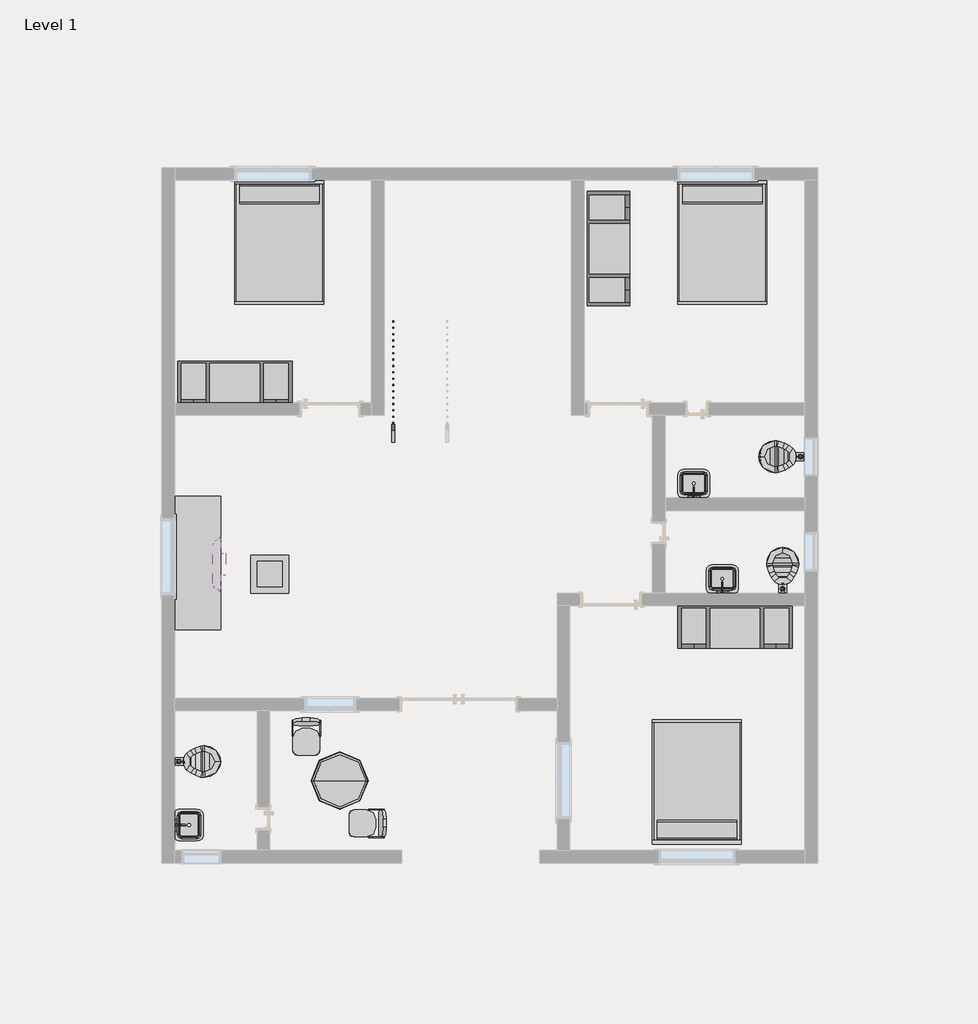
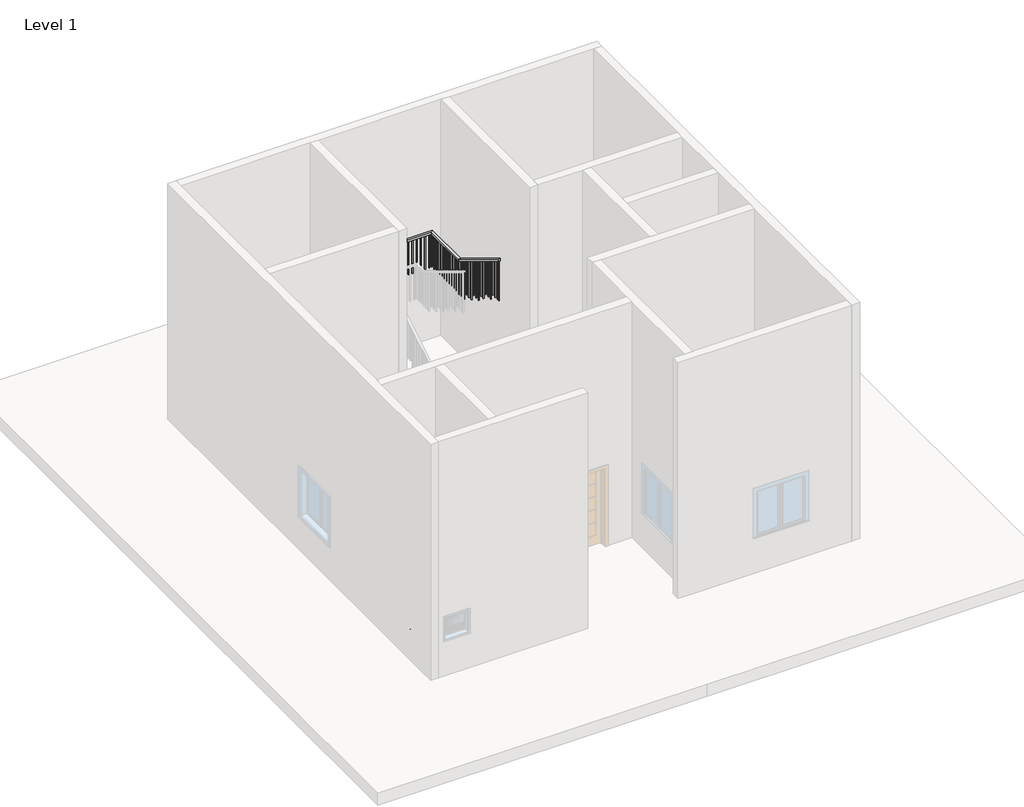
# One storey, part 3 of 3: 12 furniture elements, 6 flow terminals, 1 railing.
"""IFC4 building model written with IfcOpenShell, lengths in millimetres."""

from ifc_helpers import new_model, si_unit, frame, origin, place, context, project, spatial, polyline, outline, extrude, faceted_brep, transform, mapped, element, save
from components import flow_terminal_62a433f7, flow_terminal_bd37145e, furniture_096e7f55, furniture_cf0b6580, furniture_3d1d9cbc, furniture_56245f3a, furniture_b5c51a22, furniture_92191dda, furniture_c80d6d9c

model = new_model("IFC4")

# Units and contexts
model_context = context("Model", 3, world=origin())
ifc_project = project(units=[si_unit("LENGTHUNIT", "METRE", prefix="MILLI")], contexts=[model_context])

# Site, building, storey
site = spatial("IfcSite", under=ifc_project)
building = spatial("IfcBuilding", under=site)
storey = spatial("IfcBuildingStorey", under=building, Name="Level 1", Elevation=0.0)

# Flow terminals
placement = place(None, origin())
flow_terminal_shape = flow_terminal_62a433f7(model_context)
element("IfcFlowTerminal", 1, ObjectType="Sink Vanity-Square : 20\" x 18\"", at=placement, inside=storey, context=model_context, shape_type="MappedRepresentation", body=[
    mapped(flow_terminal_shape, transform((-11513.3414158, 2337.5597862, 0.0), x_axis=(0.0, 1.0000000000000002, 0.0), y_axis=(-1.0000000000000002, 0.0, 0.0), z_axis=(0.0, 0.0, 1.0))),
])
element("IfcFlowTerminal", 2, ObjectType="Sink Vanity-Square : 20\" x 18\"", at=placement, inside=storey, context=model_context, shape_type="MappedRepresentation", body=[
    mapped(flow_terminal_shape, transform((-3371.9975763, 7765.7944279, 0.0), x_axis=(-1.0000000000000004, 0.0, 0.0), y_axis=(0.0, -1.0000000000000004, 0.0), z_axis=(0.0, 0.0, 1.0))),
])
element("IfcFlowTerminal", 3, ObjectType="Sink Vanity-Square : 20\" x 18\"", at=placement, inside=storey, context=model_context, shape_type="MappedRepresentation", body=[
    mapped(flow_terminal_shape, transform((-2914.7975763, 6241.7944279, 0.0), x_axis=(-1.0, 0.0, 0.0), y_axis=(0.0, -1.0, 0.0), z_axis=(0.0, 0.0, 1.0))),
])
flow_terminal_2_shape = flow_terminal_bd37145e(model_context)
element("IfcFlowTerminal", 4, ObjectType="Toilet-Commercial-Wall-3D : 15\" Seat Height", at=placement, inside=storey, context=model_context, shape_type="MappedRepresentation", body=[
    mapped(flow_terminal_2_shape, transform((-1508.0868169, 7841.1458729, 0.0), x_axis=(0.0, 1.0, 0.0), y_axis=(-1.0, 0.0, 0.0), z_axis=(0.0, 0.0, 1.0))),
])
element("IfcFlowTerminal", 5, ObjectType="Toilet-Commercial-Wall-3D : 15\" Seat Height", at=placement, inside=storey, context=model_context, shape_type="MappedRepresentation", body=[
    mapped(flow_terminal_2_shape, transform((-2370.1899707, 5960.0490268, 0.0), x_axis=(1.0, 0.0, 0.0), y_axis=(0.0, 1.0, 0.0), z_axis=(0.0, 0.0, 1.0))),
])
element("IfcFlowTerminal", 6, ObjectType="Toilet-Commercial-Wall-3D : 15\" Seat Height", at=placement, inside=storey, context=model_context, shape_type="MappedRepresentation", body=[
    mapped(flow_terminal_2_shape, transform((-11795.0868169, 3774.1521806, 0.0), x_axis=(0.0, -1.0, 0.0), y_axis=(1.0, 0.0, 0.0), z_axis=(0.0, 0.0, 1.0))),
])

# Furniture
furniture_shape = furniture_096e7f55(model_context)
element("IfcFurniture", 7, ObjectType="Bed-Shaker : Double 56\" x 78\"", at=placement, inside=storey, context=model_context, shape_type="MappedRepresentation", body=[
    mapped(furniture_shape, transform((-9998.0368169, 12665.6490268, 0.0), x_axis=(1.0, 0.0, 0.0), y_axis=(0.0, 1.0, 0.0), z_axis=(0.0, 0.0, 1.0))),
])
element("IfcFurniture", 8, ObjectType="Bed-Shaker : Double 56\" x 78\"", at=placement, inside=storey, context=model_context, shape_type="MappedRepresentation", body=[
    mapped(furniture_shape, transform((-2911.4368169, 12665.6490268, 0.0), x_axis=(1.0, 0.0, 0.0), y_axis=(0.0, 1.0, 0.0), z_axis=(0.0, 0.0, 1.0))),
])
element("IfcFurniture", 9, ObjectType="Bed-Shaker : Double 56\" x 78\"", at=placement, inside=storey, context=model_context, shape_type="MappedRepresentation", body=[
    mapped(furniture_shape, transform((-3355.9368169, 2056.4587448, 0.0), x_axis=(-1.0, 0.0, 0.0), y_axis=(0.0, -1.0, 0.0), z_axis=(0.0, 0.0, 1.0))),
])
furniture_2_shape = furniture_cf0b6580(model_context)
element("IfcFurniture", 10, ObjectType="Entertainment Center : 72\" x 72\" x 24\"", at=placement, inside=storey, context=model_context, shape_type="MappedRepresentation", body=[
    mapped(furniture_2_shape, transform((-10728.2868169, 9871.6490268, 0.0), x_axis=(1.0, 0.0, 0.0), y_axis=(0.0, 1.0, 0.0), z_axis=(0.0, 0.0, 1.0))),
])
element("IfcFurniture", 11, ObjectType="Entertainment Center : 72\" x 72\" x 24\"", at=placement, inside=storey, context=model_context, shape_type="MappedRepresentation", body=[
    mapped(furniture_2_shape, transform((-5191.0868169, 11573.4490268, 0.0), x_axis=(0.0, 1.0, 0.0), y_axis=(-1.0, 0.0, 0.0), z_axis=(0.0, 0.0, 1.0))),
])
element("IfcFurniture", 12, ObjectType="Entertainment Center : 72\" x 72\" x 24\"", at=placement, inside=storey, context=model_context, shape_type="MappedRepresentation", body=[
    mapped(furniture_2_shape, transform((-2727.2868169, 5960.0490268, 0.0), x_axis=(1.0, 0.0, 0.0), y_axis=(0.0, 1.0, 0.0), z_axis=(0.0, 0.0, 1.0))),
])
furniture_3_shape = furniture_3d1d9cbc(model_context)
element("IfcFurniture", 13, ObjectType="Seating-Auditorium : 18\" x 24\" x 30\"", at=placement, inside=storey, context=model_context, shape_type="MappedRepresentation", body=[
    mapped(furniture_3_shape, transform((-9424.558948, 3965.5244366, 0.0), x_axis=(-1.0000000000000009, 0.0, 0.0), y_axis=(0.0, -1.0000000000000009, 0.0), z_axis=(0.0, 0.0, 1.0))),
])
element("IfcFurniture", 14, ObjectType="Seating-Auditorium : 18\" x 24\" x 30\"", at=placement, inside=storey, context=model_context, shape_type="MappedRepresentation", body=[
    mapped(furniture_3_shape, transform((-8404.811407, 2217.9211579, 0.0), x_axis=(0.0, 1.0000000000000004, 0.0), y_axis=(-1.0000000000000004, 0.0, 0.0), z_axis=(0.0, 0.0, 1.0))),
])
furniture_4_shape = furniture_56245f3a(model_context)
element("IfcFurniture", 15, ObjectType="TV - Flat Screen : 32\"", at=placement, inside=storey, context=model_context, shape_type="MappedRepresentation", body=[
    mapped(furniture_4_shape, transform((-11026.3147399, 6526.0559822, 1219.2), x_axis=(0.0, 1.0000000000000009, 0.0), y_axis=(-1.0000000000000009, 0.0, 0.0), z_axis=(0.0, 0.0, 1.0))),
])
furniture_5_shape = furniture_b5c51a22(model_context)
element("IfcFurniture", 16, ObjectType="Table-Coffee : 24\" x 24\" x 24\"", at=placement, inside=storey, context=model_context, shape_type="MappedRepresentation", body=[
    mapped(furniture_5_shape, transform((-10074.2757391, 6348.1832601, 0.0), x_axis=(0.0, 1.0000000000000002, 0.0), y_axis=(-1.0000000000000002, 0.0, 0.0), z_axis=(0.0, 0.0, 1.0))),
])
furniture_6_shape = furniture_92191dda(model_context)
element("IfcFurniture", 17, ObjectType="Table-Dining : 30\" x 84\" x 22\"", at=placement, inside=storey, context=model_context, shape_type="MappedRepresentation", body=[
    mapped(furniture_6_shape, transform((-11242.6757391, 6525.9832601, 0.0), x_axis=(0.0, 1.0, 0.0), y_axis=(-1.0, 0.0, 0.0), z_axis=(0.0, 0.0, 1.0))),
])
furniture_7_shape = furniture_c80d6d9c(model_context)
element("IfcFurniture", 18, ObjectType="Table-Round : 36\" Diameter", at=placement, inside=storey, context=model_context, shape_type="MappedRepresentation", body=[
    mapped(furniture_7_shape, transform((-9051.8868169, 3064.4490268, 0.0), x_axis=(1.0, 0.0, 0.0), y_axis=(0.0, 1.0, 0.0), z_axis=(0.0, 0.0, 1.0))),
])

# Railing
element("IfcRailing", 19, ObjectType="Handrail - Rectangular", at=placement, inside=storey, context=model_context, shape_type="SolidModel", body=[
    faceted_brep([(-8219.6582637, 8478.2414332, 1083.7333333), (-8219.6582637, 8478.2414332, 1024.3318731), (-8168.8582637, 8478.2414332, 1024.3318731), (-8168.8582637, 8478.2414332, 1083.7333333), (-8219.6582637, 11551.6414332, 2946.4), (-8219.6582637, 11565.8338426, 2895.6), (-8168.8582637, 11565.8338426, 2895.6), (-8168.8582637, 11551.6414332, 2946.4), (-8219.6582637, 12466.0414332, 2946.4), (-8219.6582637, 12466.0414332, 2895.6), (-8168.8582637, 12415.2414332, 2895.6), (-8168.8582637, 12415.2414332, 2946.4), (-5664.5029886, 12466.0414332, 2946.4), (-5664.5029886, 12466.0414332, 2895.6), (-5715.3029886, 12415.2414332, 2895.6), (-5715.3029886, 12415.2414332, 2946.4), (-5664.5029886, 11272.2414332, 2946.4), (-5664.5029886, 11258.0490238, 2895.6), (-5715.3029886, 11258.0490238, 2895.6), (-5715.3029886, 11272.2414332, 2946.4), (-5664.5029886, 9595.8414332, 3962.4), (-5715.3029886, 9595.8414332, 3962.4), (-5715.3029886, 9595.8414332, 3902.9985397), (-5664.5029886, 9595.8414332, 3902.9985397)], [[[0, 1, 2, 3]], [[1, 0, 4, 5]], [[2, 1, 5, 6]], [[3, 2, 6, 7]], [[0, 3, 7, 4]], [[5, 4, 8, 9]], [[6, 5, 9, 10]], [[7, 6, 10, 11]], [[4, 7, 11, 8]], [[9, 8, 12, 13]], [[10, 9, 13, 14]], [[11, 10, 14, 15]], [[8, 11, 15, 12]], [[13, 12, 16, 17]], [[14, 13, 17, 18]], [[15, 14, 18, 19]], [[12, 15, 19, 16]], [[20, 21, 22, 23]], [[17, 16, 20, 23]], [[18, 17, 23, 22]], [[19, 18, 22, 21]], [[16, 19, 21, 20]]]),
    extrude(outline(polyline([(9656.1664332, 3866.4379337), (9656.1664332, 2878.6666667), (9637.1164332, 2878.6666667), (9637.1164332, 3877.9833882), (9656.1664332, 3866.4379337)])), frame((-5699.4279886, 0.0, 0.0), z_axis=(1.0, 0.0, 0.0), x_axis=(0.0, 1.0, 0.0)), (0.0, 0.0, 1.0), 19.05),
    extrude(outline(polyline([(9757.7664332, 3804.8621761), (9757.7664332, 2878.6666667), (9738.7164332, 2878.6666667), (9738.7164332, 3816.4076307), (9757.7664332, 3804.8621761)])), frame((-5699.4279886, 0.0, 0.0), z_axis=(1.0, 0.0, 0.0), x_axis=(0.0, 1.0, 0.0)), (0.0, 0.0, 1.0), 19.05),
    extrude(outline(polyline([(9859.3664332, 3743.2864185), (9859.3664332, 2878.6666667), (9840.3164332, 2878.6666667), (9840.3164332, 3754.8318731), (9859.3664332, 3743.2864185)])), frame((-5699.4279886, 0.0, 0.0), z_axis=(1.0, 0.0, 0.0), x_axis=(0.0, 1.0, 0.0)), (0.0, 0.0, 1.0), 19.05),
    extrude(outline(polyline([(9960.9664332, 3681.710661), (9960.9664332, 2709.3333333), (9941.9164332, 2709.3333333), (9941.9164332, 3693.2561155), (9960.9664332, 3681.710661)])), frame((-5699.4279886, 0.0, 0.0), z_axis=(1.0, 0.0, 0.0), x_axis=(0.0, 1.0, 0.0)), (0.0, 0.0, 1.0), 19.05),
    extrude(outline(polyline([(10062.5664332, 3620.1349034), (10062.5664332, 2709.3333333), (10043.5164332, 2709.3333333), (10043.5164332, 3631.6803579), (10062.5664332, 3620.1349034)])), frame((-5699.4279886, 0.0, 0.0), z_axis=(1.0, 0.0, 0.0), x_axis=(0.0, 1.0, 0.0)), (0.0, 0.0, 1.0), 19.05),
    extrude(outline(polyline([(10164.1664332, 3558.5591458), (10164.1664332, 2709.3333333), (10145.1164332, 2709.3333333), (10145.1164332, 3570.1046004), (10164.1664332, 3558.5591458)])), frame((-5699.4279886, 0.0, 0.0), z_axis=(1.0, 0.0, 0.0), x_axis=(0.0, 1.0, 0.0)), (0.0, 0.0, 1.0), 19.05),
    extrude(outline(polyline([(10265.7664332, 3496.9833882), (10265.7664332, 2540.0), (10246.7164332, 2540.0), (10246.7164332, 3508.5288428), (10265.7664332, 3496.9833882)])), frame((-5699.4279886, 0.0, 0.0), z_axis=(1.0, 0.0, 0.0), x_axis=(0.0, 1.0, 0.0)), (0.0, 0.0, 1.0), 19.05),
    extrude(outline(polyline([(10367.3664332, 3435.4076307), (10367.3664332, 2540.0), (10348.3164332, 2540.0), (10348.3164332, 3446.9530852), (10367.3664332, 3435.4076307)])), frame((-5699.4279886, 0.0, 0.0), z_axis=(1.0, 0.0, 0.0), x_axis=(0.0, 1.0, 0.0)), (0.0, 0.0, 1.0), 19.05),
    extrude(outline(polyline([(10468.9664332, 3373.8318731), (10468.9664332, 2370.6666667), (10449.9164332, 2370.6666667), (10449.9164332, 3385.3773276), (10468.9664332, 3373.8318731)])), frame((-5699.4279886, 0.0, 0.0), z_axis=(1.0, 0.0, 0.0), x_axis=(0.0, 1.0, 0.0)), (0.0, 0.0, 1.0), 19.05),
    extrude(outline(polyline([(10570.5664332, 3312.2561155), (10570.5664332, 2370.6666667), (10551.5164332, 2370.6666667), (10551.5164332, 3323.80157), (10570.5664332, 3312.2561155)])), frame((-5699.4279886, 0.0, 0.0), z_axis=(1.0, 0.0, 0.0), x_axis=(0.0, 1.0, 0.0)), (0.0, 0.0, 1.0), 19.05),
    extrude(outline(polyline([(10672.1664332, 3250.6803579), (10672.1664332, 2370.6666667), (10653.1164332, 2370.6666667), (10653.1164332, 3262.2258125), (10672.1664332, 3250.6803579)])), frame((-5699.4279886, 0.0, 0.0), z_axis=(1.0, 0.0, 0.0), x_axis=(0.0, 1.0, 0.0)), (0.0, 0.0, 1.0), 19.05),
    extrude(outline(polyline([(10773.7664332, 3189.1046004), (10773.7664332, 2201.3333333), (10754.7164332, 2201.3333333), (10754.7164332, 3200.6500549), (10773.7664332, 3189.1046004)])), frame((-5699.4279886, 0.0, 0.0), z_axis=(1.0, 0.0, 0.0), x_axis=(0.0, 1.0, 0.0)), (0.0, 0.0, 1.0), 19.05),
    extrude(outline(polyline([(10875.3664332, 3127.5288428), (10875.3664332, 2201.3333333), (10856.3164332, 2201.3333333), (10856.3164332, 3139.0742973), (10875.3664332, 3127.5288428)])), frame((-5699.4279886, 0.0, 0.0), z_axis=(1.0, 0.0, 0.0), x_axis=(0.0, 1.0, 0.0)), (0.0, 0.0, 1.0), 19.05),
    extrude(outline(polyline([(10976.9664332, 3065.9530852), (10976.9664332, 2201.3333333), (10957.9164332, 2201.3333333), (10957.9164332, 3077.4985397), (10976.9664332, 3065.9530852)])), frame((-5699.4279886, 0.0, 0.0), z_axis=(1.0, 0.0, 0.0), x_axis=(0.0, 1.0, 0.0)), (0.0, 0.0, 1.0), 19.05),
    extrude(outline(polyline([(11078.5664332, 3004.3773276), (11078.5664332, 2032.0), (11059.5164332, 2032.0), (11059.5164332, 3015.9227822), (11078.5664332, 3004.3773276)])), frame((-5699.4279886, 0.0, 0.0), z_axis=(1.0, 0.0, 0.0), x_axis=(0.0, 1.0, 0.0)), (0.0, 0.0, 1.0), 19.05),
    extrude(outline(polyline([(11180.1664332, 2942.80157), (11180.1664332, 2032.0), (11161.1164332, 2032.0), (11161.1164332, 2954.3470246), (11180.1664332, 2942.80157)])), frame((-5699.4279886, 0.0, 0.0), z_axis=(1.0, 0.0, 0.0), x_axis=(0.0, 1.0, 0.0)), (0.0, 0.0, 1.0), 19.05),
    extrude(outline(polyline([(-5680.3779886, 11332.5664332), (-5680.3779886, 11313.5164332), (-5699.4279886, 11313.5164332), (-5699.4279886, 11332.5664332), (-5680.3779886, 11332.5664332)])), frame((0.0, 0.0, 2032.0), z_axis=(0.0, 0.0, 1.0), x_axis=(1.0, 0.0, 0.0)), (0.0, 0.0, 1.0), 863.6),
    extrude(outline(polyline([(-5680.3779886, 11434.1664332), (-5680.3779886, 11415.1164332), (-5699.4279886, 11415.1164332), (-5699.4279886, 11434.1664332), (-5680.3779886, 11434.1664332)])), frame((0.0, 0.0, 2032.0), z_axis=(0.0, 0.0, 1.0), x_axis=(1.0, 0.0, 0.0)), (0.0, 0.0, 1.0), 863.6),
    extrude(outline(polyline([(-5680.3779886, 11535.7664332), (-5680.3779886, 11516.7164332), (-5699.4279886, 11516.7164332), (-5699.4279886, 11535.7664332), (-5680.3779886, 11535.7664332)])), frame((0.0, 0.0, 2032.0), z_axis=(0.0, 0.0, 1.0), x_axis=(1.0, 0.0, 0.0)), (0.0, 0.0, 1.0), 863.6),
    extrude(outline(polyline([(-5680.3779886, 11637.3664332), (-5680.3779886, 11618.3164332), (-5699.4279886, 11618.3164332), (-5699.4279886, 11637.3664332), (-5680.3779886, 11637.3664332)])), frame((0.0, 0.0, 2032.0), z_axis=(0.0, 0.0, 1.0), x_axis=(1.0, 0.0, 0.0)), (0.0, 0.0, 1.0), 863.6),
    extrude(outline(polyline([(-5680.3779886, 11738.9664332), (-5680.3779886, 11719.9164332), (-5699.4279886, 11719.9164332), (-5699.4279886, 11738.9664332), (-5680.3779886, 11738.9664332)])), frame((0.0, 0.0, 2032.0), z_axis=(0.0, 0.0, 1.0), x_axis=(1.0, 0.0, 0.0)), (0.0, 0.0, 1.0), 863.6),
    extrude(outline(polyline([(-5680.3779886, 11840.5664332), (-5680.3779886, 11821.5164332), (-5699.4279886, 11821.5164332), (-5699.4279886, 11840.5664332), (-5680.3779886, 11840.5664332)])), frame((0.0, 0.0, 2032.0), z_axis=(0.0, 0.0, 1.0), x_axis=(1.0, 0.0, 0.0)), (0.0, 0.0, 1.0), 863.6),
    extrude(outline(polyline([(-5680.3779886, 11942.1664332), (-5680.3779886, 11923.1164332), (-5699.4279886, 11923.1164332), (-5699.4279886, 11942.1664332), (-5680.3779886, 11942.1664332)])), frame((0.0, 0.0, 2032.0), z_axis=(0.0, 0.0, 1.0), x_axis=(1.0, 0.0, 0.0)), (0.0, 0.0, 1.0), 863.6),
    extrude(outline(polyline([(-5680.3779886, 12043.7664332), (-5680.3779886, 12024.7164332), (-5699.4279886, 12024.7164332), (-5699.4279886, 12043.7664332), (-5680.3779886, 12043.7664332)])), frame((0.0, 0.0, 2032.0), z_axis=(0.0, 0.0, 1.0), x_axis=(1.0, 0.0, 0.0)), (0.0, 0.0, 1.0), 863.6),
    extrude(outline(polyline([(-5680.3779886, 12145.3664332), (-5680.3779886, 12126.3164332), (-5699.4279886, 12126.3164332), (-5699.4279886, 12145.3664332), (-5680.3779886, 12145.3664332)])), frame((0.0, 0.0, 2032.0), z_axis=(0.0, 0.0, 1.0), x_axis=(1.0, 0.0, 0.0)), (0.0, 0.0, 1.0), 863.6),
    extrude(outline(polyline([(-5680.3779886, 12246.9664332), (-5680.3779886, 12227.9164332), (-5699.4279886, 12227.9164332), (-5699.4279886, 12246.9664332), (-5680.3779886, 12246.9664332)])), frame((0.0, 0.0, 2032.0), z_axis=(0.0, 0.0, 1.0), x_axis=(1.0, 0.0, 0.0)), (0.0, 0.0, 1.0), 863.6),
    extrude(outline(polyline([(-5680.3779886, 12348.5664332), (-5680.3779886, 12329.5164332), (-5699.4279886, 12329.5164332), (-5699.4279886, 12348.5664332), (-5680.3779886, 12348.5664332)])), frame((0.0, 0.0, 2032.0), z_axis=(0.0, 0.0, 1.0), x_axis=(1.0, 0.0, 0.0)), (0.0, 0.0, 1.0), 863.6),
    extrude(outline(polyline([(-5765.3832637, 12450.1664332), (-5746.3332637, 12450.1664332), (-5746.3332637, 12431.1164332), (-5765.3832637, 12431.1164332), (-5765.3832637, 12450.1664332)])), frame((0.0, 0.0, 2032.0), z_axis=(0.0, 0.0, 1.0), x_axis=(1.0, 0.0, 0.0)), (0.0, 0.0, 1.0), 863.6),
    extrude(outline(polyline([(-5866.9832637, 12450.1664332), (-5847.9332637, 12450.1664332), (-5847.9332637, 12431.1164332), (-5866.9832637, 12431.1164332), (-5866.9832637, 12450.1664332)])), frame((0.0, 0.0, 2032.0), z_axis=(0.0, 0.0, 1.0), x_axis=(1.0, 0.0, 0.0)), (0.0, 0.0, 1.0), 863.6),
    extrude(outline(polyline([(-5968.5832637, 12450.1664332), (-5949.5332637, 12450.1664332), (-5949.5332637, 12431.1164332), (-5968.5832637, 12431.1164332), (-5968.5832637, 12450.1664332)])), frame((0.0, 0.0, 2032.0), z_axis=(0.0, 0.0, 1.0), x_axis=(1.0, 0.0, 0.0)), (0.0, 0.0, 1.0), 863.6),
    extrude(outline(polyline([(-6070.1832637, 12450.1664332), (-6051.1332637, 12450.1664332), (-6051.1332637, 12431.1164332), (-6070.1832637, 12431.1164332), (-6070.1832637, 12450.1664332)])), frame((0.0, 0.0, 2032.0), z_axis=(0.0, 0.0, 1.0), x_axis=(1.0, 0.0, 0.0)), (0.0, 0.0, 1.0), 863.6),
    extrude(outline(polyline([(-6171.7832637, 12450.1664332), (-6152.7332637, 12450.1664332), (-6152.7332637, 12431.1164332), (-6171.7832637, 12431.1164332), (-6171.7832637, 12450.1664332)])), frame((0.0, 0.0, 2032.0), z_axis=(0.0, 0.0, 1.0), x_axis=(1.0, 0.0, 0.0)), (0.0, 0.0, 1.0), 863.6),
    extrude(outline(polyline([(-6273.3832637, 12450.1664332), (-6254.3332637, 12450.1664332), (-6254.3332637, 12431.1164332), (-6273.3832637, 12431.1164332), (-6273.3832637, 12450.1664332)])), frame((0.0, 0.0, 2032.0), z_axis=(0.0, 0.0, 1.0), x_axis=(1.0, 0.0, 0.0)), (0.0, 0.0, 1.0), 863.6),
    extrude(outline(polyline([(-6374.9832637, 12450.1664332), (-6355.9332637, 12450.1664332), (-6355.9332637, 12431.1164332), (-6374.9832637, 12431.1164332), (-6374.9832637, 12450.1664332)])), frame((0.0, 0.0, 2032.0), z_axis=(0.0, 0.0, 1.0), x_axis=(1.0, 0.0, 0.0)), (0.0, 0.0, 1.0), 863.6),
    extrude(outline(polyline([(-6476.5832637, 12450.1664332), (-6457.5332637, 12450.1664332), (-6457.5332637, 12431.1164332), (-6476.5832637, 12431.1164332), (-6476.5832637, 12450.1664332)])), frame((0.0, 0.0, 2032.0), z_axis=(0.0, 0.0, 1.0), x_axis=(1.0, 0.0, 0.0)), (0.0, 0.0, 1.0), 863.6),
    extrude(outline(polyline([(-6578.1832637, 12450.1664332), (-6559.1332637, 12450.1664332), (-6559.1332637, 12431.1164332), (-6578.1832637, 12431.1164332), (-6578.1832637, 12450.1664332)])), frame((0.0, 0.0, 2032.0), z_axis=(0.0, 0.0, 1.0), x_axis=(1.0, 0.0, 0.0)), (0.0, 0.0, 1.0), 863.6),
    extrude(outline(polyline([(-6679.7832637, 12450.1664332), (-6660.7332637, 12450.1664332), (-6660.7332637, 12431.1164332), (-6679.7832637, 12431.1164332), (-6679.7832637, 12450.1664332)])), frame((0.0, 0.0, 2032.0), z_axis=(0.0, 0.0, 1.0), x_axis=(1.0, 0.0, 0.0)), (0.0, 0.0, 1.0), 863.6),
    extrude(outline(polyline([(-6781.3832637, 12450.1664332), (-6762.3332637, 12450.1664332), (-6762.3332637, 12431.1164332), (-6781.3832637, 12431.1164332), (-6781.3832637, 12450.1664332)])), frame((0.0, 0.0, 2032.0), z_axis=(0.0, 0.0, 1.0), x_axis=(1.0, 0.0, 0.0)), (0.0, 0.0, 1.0), 863.6),
    extrude(outline(polyline([(-6882.9832637, 12450.1664332), (-6863.9332637, 12450.1664332), (-6863.9332637, 12431.1164332), (-6882.9832637, 12431.1164332), (-6882.9832637, 12450.1664332)])), frame((0.0, 0.0, 2032.0), z_axis=(0.0, 0.0, 1.0), x_axis=(1.0, 0.0, 0.0)), (0.0, 0.0, 1.0), 863.6),
    extrude(outline(polyline([(-6984.5832637, 12450.1664332), (-6965.5332637, 12450.1664332), (-6965.5332637, 12431.1164332), (-6984.5832637, 12431.1164332), (-6984.5832637, 12450.1664332)])), frame((0.0, 0.0, 2032.0), z_axis=(0.0, 0.0, 1.0), x_axis=(1.0, 0.0, 0.0)), (0.0, 0.0, 1.0), 863.6),
    extrude(outline(polyline([(-7086.1832637, 12450.1664332), (-7067.1332637, 12450.1664332), (-7067.1332637, 12431.1164332), (-7086.1832637, 12431.1164332), (-7086.1832637, 12450.1664332)])), frame((0.0, 0.0, 2032.0), z_axis=(0.0, 0.0, 1.0), x_axis=(1.0, 0.0, 0.0)), (0.0, 0.0, 1.0), 863.6),
    extrude(outline(polyline([(-7187.7832637, 12450.1664332), (-7168.7332637, 12450.1664332), (-7168.7332637, 12431.1164332), (-7187.7832637, 12431.1164332), (-7187.7832637, 12450.1664332)])), frame((0.0, 0.0, 2032.0), z_axis=(0.0, 0.0, 1.0), x_axis=(1.0, 0.0, 0.0)), (0.0, 0.0, 1.0), 863.6),
    extrude(outline(polyline([(-7289.3832637, 12450.1664332), (-7270.3332637, 12450.1664332), (-7270.3332637, 12431.1164332), (-7289.3832637, 12431.1164332), (-7289.3832637, 12450.1664332)])), frame((0.0, 0.0, 2032.0), z_axis=(0.0, 0.0, 1.0), x_axis=(1.0, 0.0, 0.0)), (0.0, 0.0, 1.0), 863.6),
    extrude(outline(polyline([(-7390.9832637, 12450.1664332), (-7371.9332637, 12450.1664332), (-7371.9332637, 12431.1164332), (-7390.9832637, 12431.1164332), (-7390.9832637, 12450.1664332)])), frame((0.0, 0.0, 2032.0), z_axis=(0.0, 0.0, 1.0), x_axis=(1.0, 0.0, 0.0)), (0.0, 0.0, 1.0), 863.6),
    extrude(outline(polyline([(-7492.5832637, 12450.1664332), (-7473.5332637, 12450.1664332), (-7473.5332637, 12431.1164332), (-7492.5832637, 12431.1164332), (-7492.5832637, 12450.1664332)])), frame((0.0, 0.0, 2032.0), z_axis=(0.0, 0.0, 1.0), x_axis=(1.0, 0.0, 0.0)), (0.0, 0.0, 1.0), 863.6),
    extrude(outline(polyline([(-7594.1832637, 12450.1664332), (-7575.1332637, 12450.1664332), (-7575.1332637, 12431.1164332), (-7594.1832637, 12431.1164332), (-7594.1832637, 12450.1664332)])), frame((0.0, 0.0, 2032.0), z_axis=(0.0, 0.0, 1.0), x_axis=(1.0, 0.0, 0.0)), (0.0, 0.0, 1.0), 863.6),
    extrude(outline(polyline([(-7695.7832637, 12450.1664332), (-7676.7332637, 12450.1664332), (-7676.7332637, 12431.1164332), (-7695.7832637, 12431.1164332), (-7695.7832637, 12450.1664332)])), frame((0.0, 0.0, 2032.0), z_axis=(0.0, 0.0, 1.0), x_axis=(1.0, 0.0, 0.0)), (0.0, 0.0, 1.0), 863.6),
    extrude(outline(polyline([(-7797.3832637, 12450.1664332), (-7778.3332637, 12450.1664332), (-7778.3332637, 12431.1164332), (-7797.3832637, 12431.1164332), (-7797.3832637, 12450.1664332)])), frame((0.0, 0.0, 2032.0), z_axis=(0.0, 0.0, 1.0), x_axis=(1.0, 0.0, 0.0)), (0.0, 0.0, 1.0), 863.6),
    extrude(outline(polyline([(-7898.9832637, 12450.1664332), (-7879.9332637, 12450.1664332), (-7879.9332637, 12431.1164332), (-7898.9832637, 12431.1164332), (-7898.9832637, 12450.1664332)])), frame((0.0, 0.0, 2032.0), z_axis=(0.0, 0.0, 1.0), x_axis=(1.0, 0.0, 0.0)), (0.0, 0.0, 1.0), 863.6),
    extrude(outline(polyline([(-8000.5832637, 12450.1664332), (-7981.5332637, 12450.1664332), (-7981.5332637, 12431.1164332), (-8000.5832637, 12431.1164332), (-8000.5832637, 12450.1664332)])), frame((0.0, 0.0, 2032.0), z_axis=(0.0, 0.0, 1.0), x_axis=(1.0, 0.0, 0.0)), (0.0, 0.0, 1.0), 863.6),
    extrude(outline(polyline([(-8102.1832637, 12450.1664332), (-8083.1332637, 12450.1664332), (-8083.1332637, 12431.1164332), (-8102.1832637, 12431.1164332), (-8102.1832637, 12450.1664332)])), frame((0.0, 0.0, 2032.0), z_axis=(0.0, 0.0, 1.0), x_axis=(1.0, 0.0, 0.0)), (0.0, 0.0, 1.0), 863.6),
    extrude(outline(polyline([(-8203.7832637, 12354.9164332), (-8203.7832637, 12373.9664332), (-8184.7332637, 12373.9664332), (-8184.7332637, 12354.9164332), (-8203.7832637, 12354.9164332)])), frame((0.0, 0.0, 2032.0), z_axis=(0.0, 0.0, 1.0), x_axis=(1.0, 0.0, 0.0)), (0.0, 0.0, 1.0), 863.6),
    extrude(outline(polyline([(-8203.7832637, 12253.3164332), (-8203.7832637, 12272.3664332), (-8184.7332637, 12272.3664332), (-8184.7332637, 12253.3164332), (-8203.7832637, 12253.3164332)])), frame((0.0, 0.0, 2032.0), z_axis=(0.0, 0.0, 1.0), x_axis=(1.0, 0.0, 0.0)), (0.0, 0.0, 1.0), 863.6),
    extrude(outline(polyline([(-8203.7832637, 12151.7164332), (-8203.7832637, 12170.7664332), (-8184.7332637, 12170.7664332), (-8184.7332637, 12151.7164332), (-8203.7832637, 12151.7164332)])), frame((0.0, 0.0, 2032.0), z_axis=(0.0, 0.0, 1.0), x_axis=(1.0, 0.0, 0.0)), (0.0, 0.0, 1.0), 863.6),
    extrude(outline(polyline([(-8203.7832637, 12050.1164332), (-8203.7832637, 12069.1664332), (-8184.7332637, 12069.1664332), (-8184.7332637, 12050.1164332), (-8203.7832637, 12050.1164332)])), frame((0.0, 0.0, 2032.0), z_axis=(0.0, 0.0, 1.0), x_axis=(1.0, 0.0, 0.0)), (0.0, 0.0, 1.0), 863.6),
    extrude(outline(polyline([(-8203.7832637, 11948.5164332), (-8203.7832637, 11967.5664332), (-8184.7332637, 11967.5664332), (-8184.7332637, 11948.5164332), (-8203.7832637, 11948.5164332)])), frame((0.0, 0.0, 2032.0), z_axis=(0.0, 0.0, 1.0), x_axis=(1.0, 0.0, 0.0)), (0.0, 0.0, 1.0), 863.6),
    extrude(outline(polyline([(-8203.7832637, 11846.9164332), (-8203.7832637, 11865.9664332), (-8184.7332637, 11865.9664332), (-8184.7332637, 11846.9164332), (-8203.7832637, 11846.9164332)])), frame((0.0, 0.0, 2032.0), z_axis=(0.0, 0.0, 1.0), x_axis=(1.0, 0.0, 0.0)), (0.0, 0.0, 1.0), 863.6),
    extrude(outline(polyline([(-8203.7832637, 11745.3164332), (-8203.7832637, 11764.3664332), (-8184.7332637, 11764.3664332), (-8184.7332637, 11745.3164332), (-8203.7832637, 11745.3164332)])), frame((0.0, 0.0, 2032.0), z_axis=(0.0, 0.0, 1.0), x_axis=(1.0, 0.0, 0.0)), (0.0, 0.0, 1.0), 863.6),
    extrude(outline(polyline([(-8203.7832637, 11643.7164332), (-8203.7832637, 11662.7664332), (-8184.7332637, 11662.7664332), (-8184.7332637, 11643.7164332), (-8203.7832637, 11643.7164332)])), frame((0.0, 0.0, 2032.0), z_axis=(0.0, 0.0, 1.0), x_axis=(1.0, 0.0, 0.0)), (0.0, 0.0, 1.0), 863.6),
    extrude(outline(polyline([(11535.7664332, 2877.3773276), (11535.7664332, 1862.6666667), (11516.7164332, 1862.6666667), (11516.7164332, 2865.8318731), (11535.7664332, 2877.3773276)])), frame((-8203.7832637, 0.0, 0.0), z_axis=(1.0, 0.0, 0.0), x_axis=(0.0, 1.0, 0.0)), (0.0, 0.0, 1.0), 19.05),
    extrude(outline(polyline([(11434.1664332, 2815.80157), (11434.1664332, 1862.6666667), (11415.1164332, 1862.6666667), (11415.1164332, 2804.2561155), (11434.1664332, 2815.80157)])), frame((-8203.7832637, 0.0, 0.0), z_axis=(1.0, 0.0, 0.0), x_axis=(0.0, 1.0, 0.0)), (0.0, 0.0, 1.0), 19.05),
    extrude(outline(polyline([(11332.5664332, 2754.2258125), (11332.5664332, 1862.6666667), (11313.5164332, 1862.6666667), (11313.5164332, 2742.6803579), (11332.5664332, 2754.2258125)])), frame((-8203.7832637, 0.0, 0.0), z_axis=(1.0, 0.0, 0.0), x_axis=(0.0, 1.0, 0.0)), (0.0, 0.0, 1.0), 19.05),
    extrude(outline(polyline([(11230.9664332, 2692.6500549), (11230.9664332, 1693.3333333), (11211.9164332, 1693.3333333), (11211.9164332, 2681.1046004), (11230.9664332, 2692.6500549)])), frame((-8203.7832637, 0.0, 0.0), z_axis=(1.0, 0.0, 0.0), x_axis=(0.0, 1.0, 0.0)), (0.0, 0.0, 1.0), 19.05),
    extrude(outline(polyline([(11129.3664332, 2631.0742973), (11129.3664332, 1693.3333333), (11110.3164332, 1693.3333333), (11110.3164332, 2619.5288428), (11129.3664332, 2631.0742973)])), frame((-8203.7832637, 0.0, 0.0), z_axis=(1.0, 0.0, 0.0), x_axis=(0.0, 1.0, 0.0)), (0.0, 0.0, 1.0), 19.05),
    extrude(outline(polyline([(11027.7664332, 2569.4985397), (11027.7664332, 1693.3333333), (11008.7164332, 1693.3333333), (11008.7164332, 2557.9530852), (11027.7664332, 2569.4985397)])), frame((-8203.7832637, 0.0, 0.0), z_axis=(1.0, 0.0, 0.0), x_axis=(0.0, 1.0, 0.0)), (0.0, 0.0, 1.0), 19.05),
    extrude(outline(polyline([(10926.1664332, 2507.9227822), (10926.1664332, 1524.0), (10907.1164332, 1524.0), (10907.1164332, 2496.3773276), (10926.1664332, 2507.9227822)])), frame((-8203.7832637, 0.0, 0.0), z_axis=(1.0, 0.0, 0.0), x_axis=(0.0, 1.0, 0.0)), (0.0, 0.0, 1.0), 19.05),
    extrude(outline(polyline([(10824.5664332, 2446.3470246), (10824.5664332, 1524.0), (10805.5164332, 1524.0), (10805.5164332, 2434.80157), (10824.5664332, 2446.3470246)])), frame((-8203.7832637, 0.0, 0.0), z_axis=(1.0, 0.0, 0.0), x_axis=(0.0, 1.0, 0.0)), (0.0, 0.0, 1.0), 19.05),
    extrude(outline(polyline([(10722.9664332, 2384.771267), (10722.9664332, 1524.0), (10703.9164332, 1524.0), (10703.9164332, 2373.2258125), (10722.9664332, 2384.771267)])), frame((-8203.7832637, 0.0, 0.0), z_axis=(1.0, 0.0, 0.0), x_axis=(0.0, 1.0, 0.0)), (0.0, 0.0, 1.0), 19.05),
    extrude(outline(polyline([(10621.3664332, 2323.1955094), (10621.3664332, 1354.6666667), (10602.3164332, 1354.6666667), (10602.3164332, 2311.6500549), (10621.3664332, 2323.1955094)])), frame((-8203.7832637, 0.0, 0.0), z_axis=(1.0, 0.0, 0.0), x_axis=(0.0, 1.0, 0.0)), (0.0, 0.0, 1.0), 19.05),
    extrude(outline(polyline([(10519.7664332, 2261.6197519), (10519.7664332, 1354.6666667), (10500.7164332, 1354.6666667), (10500.7164332, 2250.0742973), (10519.7664332, 2261.6197519)])), frame((-8203.7832637, 0.0, 0.0), z_axis=(1.0, 0.0, 0.0), x_axis=(0.0, 1.0, 0.0)), (0.0, 0.0, 1.0), 19.05),
    extrude(outline(polyline([(10418.1664332, 2200.0439943), (10418.1664332, 1185.3333333), (10399.1164332, 1185.3333333), (10399.1164332, 2188.4985397), (10418.1664332, 2200.0439943)])), frame((-8203.7832637, 0.0, 0.0), z_axis=(1.0, 0.0, 0.0), x_axis=(0.0, 1.0, 0.0)), (0.0, 0.0, 1.0), 19.05),
    extrude(outline(polyline([(10316.5664332, 2138.4682367), (10316.5664332, 1185.3333333), (10297.5164332, 1185.3333333), (10297.5164332, 2126.9227822), (10316.5664332, 2138.4682367)])), frame((-8203.7832637, 0.0, 0.0), z_axis=(1.0, 0.0, 0.0), x_axis=(0.0, 1.0, 0.0)), (0.0, 0.0, 1.0), 19.05),
    extrude(outline(polyline([(10214.9664332, 2076.8924791), (10214.9664332, 1185.3333333), (10195.9164332, 1185.3333333), (10195.9164332, 2065.3470246), (10214.9664332, 2076.8924791)])), frame((-8203.7832637, 0.0, 0.0), z_axis=(1.0, 0.0, 0.0), x_axis=(0.0, 1.0, 0.0)), (0.0, 0.0, 1.0), 19.05),
    extrude(outline(polyline([(10113.3664332, 2015.3167216), (10113.3664332, 1016.0), (10094.3164332, 1016.0), (10094.3164332, 2003.771267), (10113.3664332, 2015.3167216)])), frame((-8203.7832637, 0.0, 0.0), z_axis=(1.0, 0.0, 0.0), x_axis=(0.0, 1.0, 0.0)), (0.0, 0.0, 1.0), 19.05),
    extrude(outline(polyline([(10011.7664332, 1953.740964), (10011.7664332, 1016.0), (9992.7164332, 1016.0), (9992.7164332, 1942.1955094), (10011.7664332, 1953.740964)])), frame((-8203.7832637, 0.0, 0.0), z_axis=(1.0, 0.0, 0.0), x_axis=(0.0, 1.0, 0.0)), (0.0, 0.0, 1.0), 19.05),
    extrude(outline(polyline([(9910.1664332, 1892.1652064), (9910.1664332, 1016.0), (9891.1164332, 1016.0), (9891.1164332, 1880.6197519), (9910.1664332, 1892.1652064)])), frame((-8203.7832637, 0.0, 0.0), z_axis=(1.0, 0.0, 0.0), x_axis=(0.0, 1.0, 0.0)), (0.0, 0.0, 1.0), 19.05),
    extrude(outline(polyline([(9808.5664332, 1830.5894488), (9808.5664332, 846.6666667), (9789.5164332, 846.6666667), (9789.5164332, 1819.0439943), (9808.5664332, 1830.5894488)])), frame((-8203.7832637, 0.0, 0.0), z_axis=(1.0, 0.0, 0.0), x_axis=(0.0, 1.0, 0.0)), (0.0, 0.0, 1.0), 19.05),
    extrude(outline(polyline([(9706.9664332, 1769.0136913), (9706.9664332, 846.6666667), (9687.9164332, 846.6666667), (9687.9164332, 1757.4682367), (9706.9664332, 1769.0136913)])), frame((-8203.7832637, 0.0, 0.0), z_axis=(1.0, 0.0, 0.0), x_axis=(0.0, 1.0, 0.0)), (0.0, 0.0, 1.0), 19.05),
    extrude(outline(polyline([(9605.3664332, 1707.4379337), (9605.3664332, 846.6666667), (9586.3164332, 846.6666667), (9586.3164332, 1695.8924791), (9605.3664332, 1707.4379337)])), frame((-8203.7832637, 0.0, 0.0), z_axis=(1.0, 0.0, 0.0), x_axis=(0.0, 1.0, 0.0)), (0.0, 0.0, 1.0), 19.05),
    extrude(outline(polyline([(9503.7664332, 1645.8621761), (9503.7664332, 677.3333333), (9484.7164332, 677.3333333), (9484.7164332, 1634.3167216), (9503.7664332, 1645.8621761)])), frame((-8203.7832637, 0.0, 0.0), z_axis=(1.0, 0.0, 0.0), x_axis=(0.0, 1.0, 0.0)), (0.0, 0.0, 1.0), 19.05),
    extrude(outline(polyline([(9402.1664332, 1584.2864185), (9402.1664332, 677.3333333), (9383.1164332, 677.3333333), (9383.1164332, 1572.740964), (9402.1664332, 1584.2864185)])), frame((-8203.7832637, 0.0, 0.0), z_axis=(1.0, 0.0, 0.0), x_axis=(0.0, 1.0, 0.0)), (0.0, 0.0, 1.0), 19.05),
    extrude(outline(polyline([(9300.5664332, 1522.710661), (9300.5664332, 508.0), (9281.5164332, 508.0), (9281.5164332, 1511.1652064), (9300.5664332, 1522.710661)])), frame((-8203.7832637, 0.0, 0.0), z_axis=(1.0, 0.0, 0.0), x_axis=(0.0, 1.0, 0.0)), (0.0, 0.0, 1.0), 19.05),
    extrude(outline(polyline([(9198.9664332, 1461.1349034), (9198.9664332, 508.0), (9179.9164332, 508.0), (9179.9164332, 1449.5894488), (9198.9664332, 1461.1349034)])), frame((-8203.7832637, 0.0, 0.0), z_axis=(1.0, 0.0, 0.0), x_axis=(0.0, 1.0, 0.0)), (0.0, 0.0, 1.0), 19.05),
    extrude(outline(polyline([(9097.3664332, 1399.5591458), (9097.3664332, 508.0), (9078.3164332, 508.0), (9078.3164332, 1388.0136913), (9097.3664332, 1399.5591458)])), frame((-8203.7832637, 0.0, 0.0), z_axis=(1.0, 0.0, 0.0), x_axis=(0.0, 1.0, 0.0)), (0.0, 0.0, 1.0), 19.05),
    extrude(outline(polyline([(8995.7664332, 1337.9833882), (8995.7664332, 338.6666667), (8976.7164332, 338.6666667), (8976.7164332, 1326.4379337), (8995.7664332, 1337.9833882)])), frame((-8203.7832637, 0.0, 0.0), z_axis=(1.0, 0.0, 0.0), x_axis=(0.0, 1.0, 0.0)), (0.0, 0.0, 1.0), 19.05),
    extrude(outline(polyline([(8894.1664332, 1276.4076307), (8894.1664332, 338.6666667), (8875.1164332, 338.6666667), (8875.1164332, 1264.8621761), (8894.1664332, 1276.4076307)])), frame((-8203.7832637, 0.0, 0.0), z_axis=(1.0, 0.0, 0.0), x_axis=(0.0, 1.0, 0.0)), (0.0, 0.0, 1.0), 19.05),
    extrude(outline(polyline([(8792.5664332, 1214.8318731), (8792.5664332, 338.6666667), (8773.5164332, 338.6666667), (8773.5164332, 1203.2864185), (8792.5664332, 1214.8318731)])), frame((-8203.7832637, 0.0, 0.0), z_axis=(1.0, 0.0, 0.0), x_axis=(0.0, 1.0, 0.0)), (0.0, 0.0, 1.0), 19.05),
    extrude(outline(polyline([(8690.9664332, 1153.2561155), (8690.9664332, 169.3333333), (8671.9164332, 169.3333333), (8671.9164332, 1141.710661), (8690.9664332, 1153.2561155)])), frame((-8203.7832637, 0.0, 0.0), z_axis=(1.0, 0.0, 0.0), x_axis=(0.0, 1.0, 0.0)), (0.0, 0.0, 1.0), 19.05),
    extrude(outline(polyline([(8589.3664332, 1091.6803579), (8589.3664332, 169.3333333), (8570.3164332, 169.3333333), (8570.3164332, 1080.1349034), (8589.3664332, 1091.6803579)])), frame((-8203.7832637, 0.0, 0.0), z_axis=(1.0, 0.0, 0.0), x_axis=(0.0, 1.0, 0.0)), (0.0, 0.0, 1.0), 19.05),
    extrude(outline(polyline([(-5680.3779886, 11281.7664332), (-5680.3779886, 11262.7164332), (-5699.4279886, 11262.7164332), (-5699.4279886, 11281.7664332), (-5680.3779886, 11281.7664332)])), frame((0.0, 0.0, 2032.0), z_axis=(0.0, 0.0, 1.0), x_axis=(1.0, 0.0, 0.0)), (0.0, 0.0, 1.0), 863.6),
    extrude(outline(polyline([(-5699.4279886, 12450.1664332), (-5680.3779886, 12450.1664332), (-5680.3779886, 12431.1164332), (-5699.4279886, 12431.1164332), (-5699.4279886, 12450.1664332)])), frame((0.0, 0.0, 2032.0), z_axis=(0.0, 0.0, 1.0), x_axis=(1.0, 0.0, 0.0)), (0.0, 0.0, 1.0), 863.6),
    extrude(outline(polyline([(-8203.7832637, 12431.1164332), (-8203.7832637, 12450.1664332), (-8184.7332637, 12450.1664332), (-8184.7332637, 12431.1164332), (-8203.7832637, 12431.1164332)])), frame((0.0, 0.0, 2032.0), z_axis=(0.0, 0.0, 1.0), x_axis=(1.0, 0.0, 0.0)), (0.0, 0.0, 1.0), 863.6),
    extrude(outline(polyline([(11561.1664332, 2892.771267), (11561.1664332, 2032.0), (11542.1164332, 2032.0), (11542.1164332, 2881.2258125), (11561.1664332, 2892.771267)])), frame((-8203.7832637, 0.0, 0.0), z_axis=(1.0, 0.0, 0.0), x_axis=(0.0, 1.0, 0.0)), (0.0, 0.0, 1.0), 19.05),
    extrude(outline(polyline([(9614.8914332, 3891.4530852), (9614.8914332, 2878.6666667), (9595.8414332, 2878.6666667), (9595.8414332, 3902.9985397), (9614.8914332, 3891.4530852)])), frame((-5699.4279886, 0.0, 0.0), z_axis=(1.0, 0.0, 0.0), x_axis=(0.0, 1.0, 0.0)), (0.0, 0.0, 1.0), 19.05),
    extrude(outline(polyline([(8497.2914332, 1035.8773276), (8497.2914332, 169.3333333), (8478.2414332, 169.3333333), (8478.2414332, 1024.3318731), (8497.2914332, 1035.8773276)])), frame((-8203.7832637, 0.0, 0.0), z_axis=(1.0, 0.0, 0.0), x_axis=(0.0, 1.0, 0.0)), (0.0, 0.0, 1.0), 19.05),
])

save(model, "model.ifc")

# Revit data of these elements
# Type "Sink Vanity-Square : 20\" x 18\""
#   Assembly Code = "D2010400"
#   Counter Height = 2' - 7"
#   Depth = 1' - 6"
#   Width = 1' - 8"
#   Basin Material = Porcelain, Linen
#   Faucet Material = Steel, Polished
#   Default Elevation = 0
# Type "Toilet-Commercial-Wall-3D : 15\" Seat Height"
#   Assembly Code = "D2010110"
#   Mounting Height = 1' - 3"
#   Piping Material = Steel, Polished
#   Toilet - Bowl Material = Porcelain, Ivory
#   Toilet - Seat Material = Laminate, Ivory, Matte
#   Default Elevation = 0
# Type "Bed-Shaker : Double 56\" x 78\""
#   Assembly Code = "E2020200"
#   Length = 6' - 6"
#   Width = 4' - 8"
#   Frame Material = Birch
#   Mattress Material = Linen, White
#   Default Elevation = 0
# Type "Entertainment Center : 72\" x 72\" x 24\""
#   Assembly Code = "E2020200"
#   Center Width = 2' - 8"
#   Depth = 2' - 0"
#   Height = 6' - 0"
#   Width = 6' - 0"
#   Material = none
#   Default Elevation = 0
# Type "Seating-Auditorium : 18\" x 24\" x 30\""
#   Assembly Code = "E2020200"
#   Seat Material = Linen, Beige
#   Frame Material = Steel, Paint Finish, Dark Gray, Matte
#   Default Elevation = 0
# Type "TV - Flat Screen : 32\""
#   SinAng = 0' - 0.0193"
#   L = 2' - 3.79372"
#   H = 1' - 3.6354"
#   Thickness = 0' - 4.33071"
#   Diagonal = 2' - 7.88976"
#   CosAng = 0' - 0.03431"
#   Stand [instance default] = yes
#   Default Elevation = 0
# Type "Table-Coffee : 24\" x 24\" x 24\""
#   Assembly Code = "E2020200"
#   Height = 2' - 0"
#   Length = 2' - 0"
#   Width = 2' - 0"
#   Top Material = none
#   Frame Material = none
#   Default Elevation = 0
# Type "Table-Dining : 30\" x 84\" x 22\""
#   Assembly Code = "E2020200"
#   Height = 1' - 10"
#   Length = 7' - 0"
#   Width = 2' - 6"
#   Base Material = Steel, Chrome Plated
#   Top Material = Glass - Clear, Grey
#   Default Elevation = 0
# Type "Table-Round : 36\" Diameter"
#   Assembly Code = "E2020200"
#   Base Radius = 0' - 10"
#   Height = 2' - 6"
#   Radius = 1' - 6"
#   Base Material = Steel, Chrome Plated
#   Top Material = Birch
#   Default Elevation = 0
# Type "Handrail - Rectangular"
#   Assembly Code = "C2010400"
#   built-in parameter 1008612 = 0.0416667 (stored number, unit not read)
#   built-in parameter 1008611 = 0.0416667 (stored number, unit not read)
#   built-in parameter 1008609 = 0.333333 (stored number, unit not read)
#   built-in parameter 1008604 = 0.166667 (stored number, unit not read)
#   built-in parameter 1008603 = 0.166667 (stored number, unit not read)
#   Railing Height = 3' - 0"
#   built-in parameter 1008630 = 2
#   built-in parameter 1008610 = 2
#   built-in parameter 1008618 = Baluster - Square : 3/4"
# Element 1 (IfcFlowTerminal, "Sink Vanity-Square : 20\" x 18\"")
#   Mark = "1"
#   Phase Created = New Construction
#   Materials on its faces: "Porcelain, Linen", "Steel, Polished"
# Element 2 (IfcFlowTerminal, "Sink Vanity-Square : 20\" x 18\"")
#   Mark = "2"
#   Phase Created = New Construction
#   Materials on its faces: "Porcelain, Linen", "Steel, Polished"
# Element 3 (IfcFlowTerminal, "Sink Vanity-Square : 20\" x 18\"")
#   Mark = "3"
#   Phase Created = New Construction
#   Materials on its faces: "Porcelain, Linen", "Steel, Polished"
# Element 4 (IfcFlowTerminal, "Toilet-Commercial-Wall-3D : 15\" Seat Height")
#   Mark = "4"
#   Phase Created = New Construction
#   Materials on its faces: "Laminate, Ivory, Matte", "Porcelain, Ivory", "Steel, Polished"
# Element 5 (IfcFlowTerminal, "Toilet-Commercial-Wall-3D : 15\" Seat Height")
#   Mark = "5"
#   Phase Created = New Construction
#   Materials on its faces: "Laminate, Ivory, Matte", "Porcelain, Ivory", "Steel, Polished"
# Element 6 (IfcFlowTerminal, "Toilet-Commercial-Wall-3D : 15\" Seat Height")
#   Mark = "6"
#   Phase Created = New Construction
#   Materials on its faces: "Laminate, Ivory, Matte", "Porcelain, Ivory", "Steel, Polished"
# Elements 7, 8, 9 (IfcFurniture, "Bed-Shaker : Double 56\" x 78\"")
#   Phase Created = New Construction
#   Materials on its faces: "Birch", "Linen, White"
# Elements 10, 11, 12 (IfcFurniture, "Entertainment Center : 72\" x 72\" x 24\"")
#   Phase Created = New Construction
#   Materials on its faces: "Steel, Chrome Plated", "Glass - Clear, Grey"
# Elements 13, 14 (IfcFurniture, "Seating-Auditorium : 18\" x 24\" x 30\"")
#   Phase Created = New Construction
#   Materials on its faces: "Steel, Paint Finish, Dark Gray, Matte", "Linen, Beige"
# Element 15 (IfcFurniture, "TV - Flat Screen : 32\"")
#   Stand = yes
#   Phase Created = New Construction
#   Materials on its faces: "TV - Black", "TV - Glass", "TV - Screen"
# Element 16 (IfcFurniture, "Table-Coffee : 24\" x 24\" x 24\"")
#   Phase Created = New Construction
#   Materials on its faces: "Glass - Clear, Grey"
# Element 17 (IfcFurniture, "Table-Dining : 30\" x 84\" x 22\"")
#   Phase Created = New Construction
#   Materials on its faces: "Steel, Chrome Plated", "Glass - Clear, Grey"
# Element 18 (IfcFurniture, "Table-Round : 36\" Diameter")
#   Phase Created = New Construction
#   Materials on its faces: "Steel, Chrome Plated", "Birch"
# Element 19 (IfcRailing, "Handrail - Rectangular")
#   Phase Created = New Construction
# Materials
#   "Porcelain, Linen": class "Ceramic", colour RGB 249 239 230, transparency 0, Description = "Porcelain, linen", Cost = 0
#   "Steel, Polished": class "Metal", colour RGB 57 57 57, transparency 0, Description = "Polished steel", Cost = 0
#   "Porcelain, Ivory": class "Ceramic", colour RGB 247 247 239, transparency 0, Description = "Porcelain, ivory", Cost = 0
#   "Laminate, Ivory, Matte": class "Plastic", colour RGB 247 247 239, transparency 0, Description = "Plastic Laminate - Ivory, Matte", Cost = 0
#   "Birch": class "Wood", colour RGB 224 178 126, transparency 0, Description = "Betula Alleghaniensis", Cost = 0
#   "Linen, White": class "Textile", colour RGB 247 247 239, transparency 0, Description = "Linen, white", Cost = 0
#   "Linen, Beige": class "Textile", colour RGB 249 239 230, transparency 0, Description = "Linen, beige", Cost = 0
#   "Steel, Paint Finish, Dark Gray, Matte": class "Metal", colour RGB 0 0 0, transparency 0, Description = "Steel, paint finish, dark gray, matte", Cost = 0
#   "Steel, Chrome Plated": class "Metal", colour RGB 17 17 17, transparency 0, Description = "Chromiuim plated steel", Cost = 0
#   "Glass - Clear, Grey": class "Glass", colour RGB 252 255 255, transparency 0.64
#   "TV - Black": colour RGB 49 49 49, transparency 0
#   "TV - Glass": colour RGB 157 157 157, transparency 0.9
#   "TV - Screen": colour RGB 0 0 0, transparency 0
